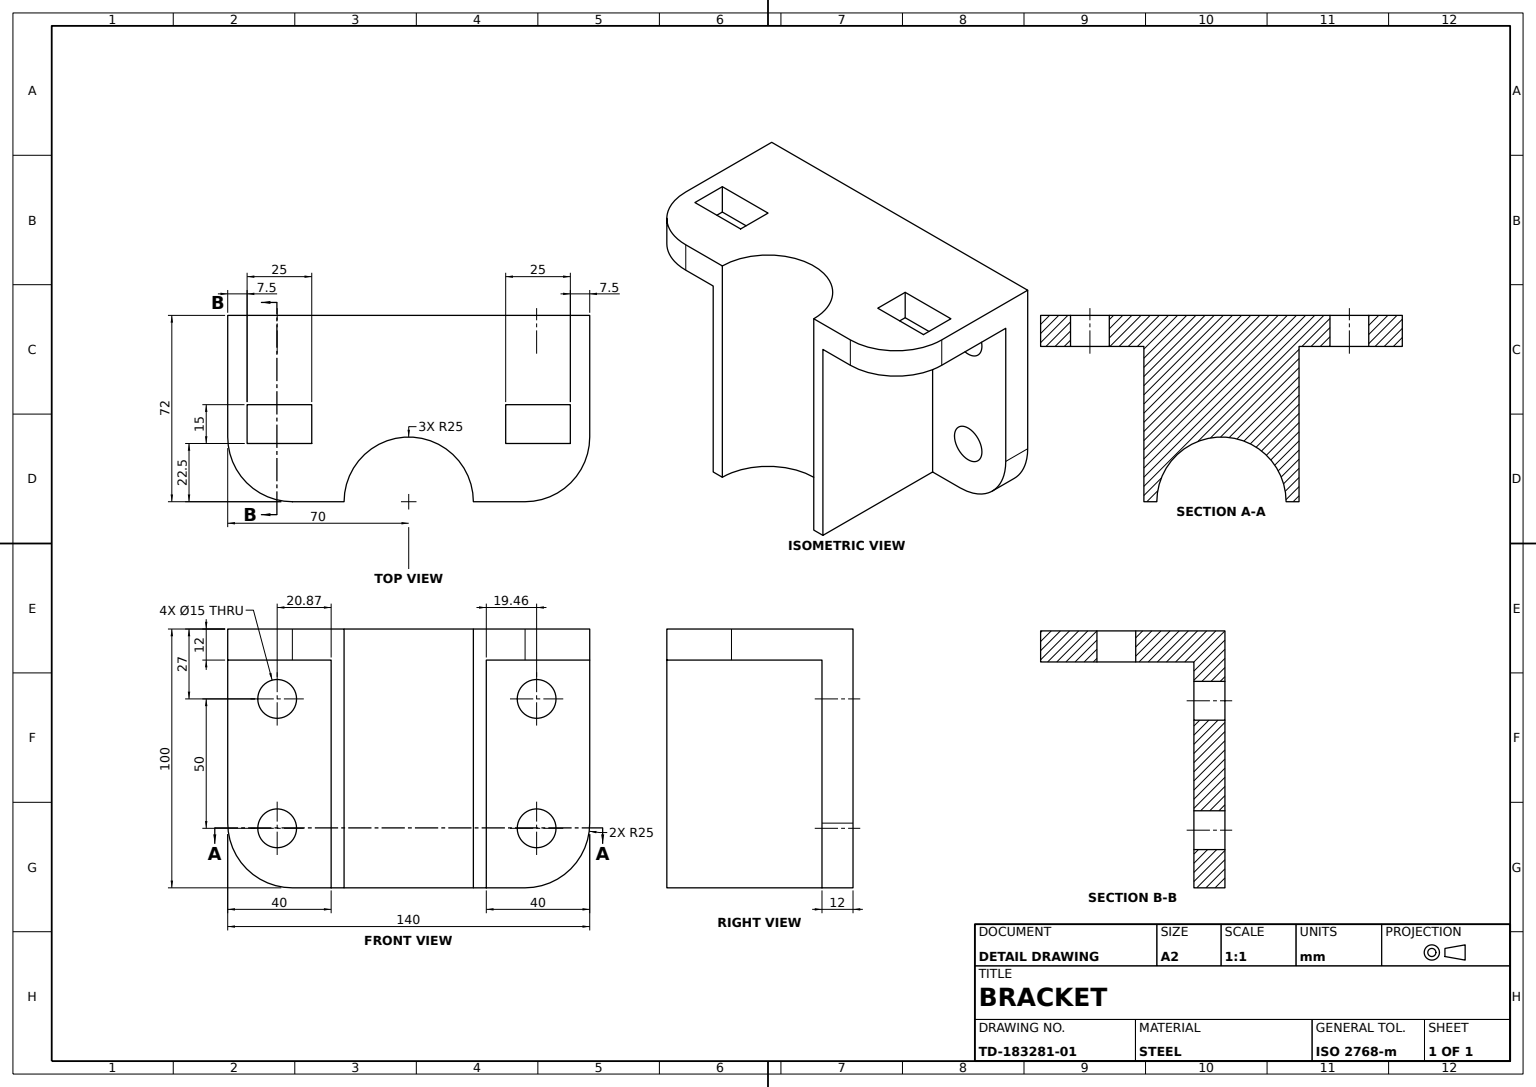
from build123d import *

# Parameters (mm, degrees)
BASE_PLATE_DEPTH         = 12
SIDE_FLANGE_DEPTH        = 12
BOSS_88MM_DEPTH          = 88
CURVED_START             = -12
CURVED_CUT_DEPTH         = 12
SLOT_A_SKETCH_22_5X7_5_W = 25
SLOT_A_SKETCH_22_5X7_5_H = 15
SLOT_A_22_5X7_5_DEPTH    = 12
SLOT_B_SKETCH_7_5X22_5_W = 25
SLOT_B_SKETCH_7_5X22_5_H = 15
SLOT_B_7_5X22_5_DEPTH    = 12
HOLE_A_SKETCH_15_R       = 7.5
HOLE_A_15_DEPTH          = 12
HOLE_B_SKETCH_15_R       = 7.5
HOLE_B_15_DEPTH          = 12


with BuildPart() as part:
    # Base Plate Sketch → Base Plate (new body)
    with BuildSketch(Plane.XY):
        with BuildLine():
            Line((0, 0), (0, -75))
            ThreePointArc((0, -75), (7.32233047, -92.67766953), (25, -100))
            Line((25, -100), (115, -100))
            ThreePointArc((115, -100), (132.67766953, -92.67766953), (140, -75))
            Line((140, -75), (140, 0))
            Line((140, 0), (0, 0))
        make_face()
    extrude(amount=BASE_PLATE_DEPTH)

    # Side Flange Sketch → Side Flange (add)
    with BuildSketch(Plane(origin=(0, 0, 0), x_dir=(1, 0, 0), z_dir=(0, 1, 0))):
        with BuildLine():
            Line((140, -12), (140, -47))
            ThreePointArc((140, -47), (132.67766953, -64.67766953), (115, -72))
            Line((115, -72), (25, -72))
            ThreePointArc((25, -72), (7.32233047, -64.67766953), (0, -47))
            Line((0, -47), (0, -12))
            Line((0, -12), (140, -12))
        make_face()
    extrude(amount=-SIDE_FLANGE_DEPTH)

    # Boss Profile Sketch → Boss 88mm (add)
    with BuildSketch(Plane.XZ.offset(12)):
        with BuildLine():
            Line((95, 72), (100, 72))
            Line((100, 72), (100, 12))
            Line((100, 12), (40, 12))
            Line((40, 12), (40, 72))
            Line((40, 72), (45, 72))
            ThreePointArc((45, 72), (70, 47), (95, 72))
        make_face()
    extrude(amount=BOSS_88MM_DEPTH)

    # Curved Cut Sketch → Curved Cut (cut)
    with BuildSketch(Plane.XZ.offset(12).offset(CURVED_START)):
        with BuildLine():
            Line((45, 72), (95, 72))
            ThreePointArc((95, 72), (70, 47), (45, 72))
        make_face()
    extrude(amount=CURVED_CUT_DEPTH, mode=Mode.SUBTRACT)

    # Slot A Sketch 22.5x7.5 → Slot A 22.5x7.5 (cut)
    with BuildSketch(Plane(origin=(0, -12, 0), x_dir=(-1, 0, 0), z_dir=(0, -1, 0))):
        with Locations((-120, -42)):
            Rectangle(SLOT_A_SKETCH_22_5X7_5_W, SLOT_A_SKETCH_22_5X7_5_H)
    extrude(amount=-SLOT_A_22_5X7_5_DEPTH, mode=Mode.SUBTRACT)

    # Slot B Sketch 7.5x22.5 → Slot B 7.5x22.5 (cut)
    with BuildSketch(Plane(origin=(0, -12, 0), x_dir=(-1, 0, 0), z_dir=(0, -1, 0))):
        with Locations((-20, -42)):
            Rectangle(SLOT_B_SKETCH_7_5X22_5_W, SLOT_B_SKETCH_7_5X22_5_H)
    extrude(amount=-SLOT_B_7_5X22_5_DEPTH, mode=Mode.SUBTRACT)

    # Hole A Sketch Ø15 → Hole A Ø15 (cut)
    with BuildSketch(Plane.XY.offset(12)):
        with Locations((119.463154548, -27)):
            Circle(HOLE_A_SKETCH_15_R)
        with Locations((119.463154548, -77)):
            Circle(HOLE_A_SKETCH_15_R)
    extrude(amount=-HOLE_A_15_DEPTH, mode=Mode.SUBTRACT)

    # Hole B Sketch Ø15 → Hole B Ø15 (cut)
    with BuildSketch(Plane.XY.offset(12)):
        with Locations((19.128084721, -27)):
            Circle(HOLE_B_SKETCH_15_R)
        with Locations((19.128084721, -77)):
            Circle(HOLE_B_SKETCH_15_R)
    extrude(amount=-HOLE_B_15_DEPTH, mode=Mode.SUBTRACT)


solid = part.part
